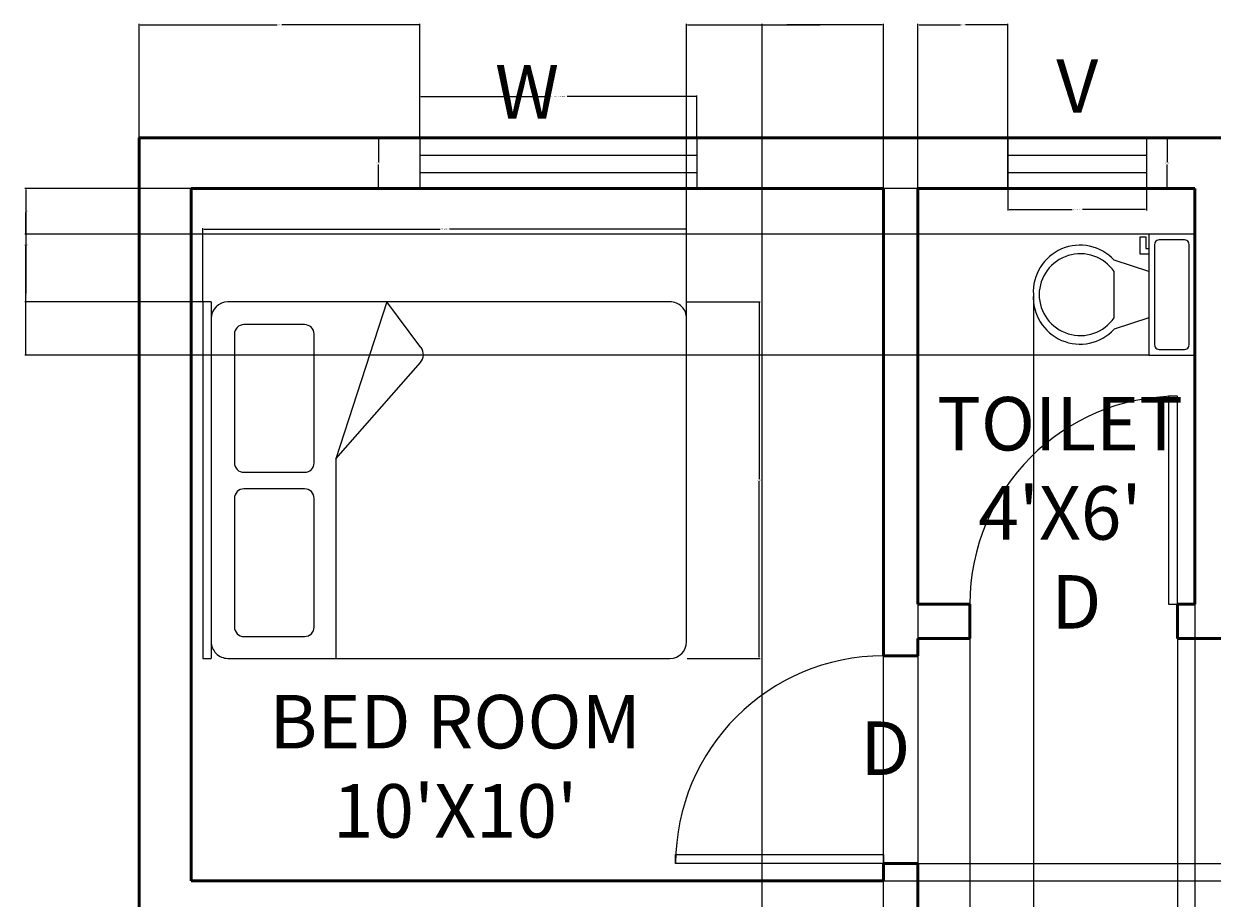
# Model space of a CAD drawing. Units: inches. Extents: x 1916 to 2328, y 785 to 1125.
# Tile 2 of 3: x 1916 to 2122, y 973 to 1125. Entities that reach past the tile are written whole.
import ezdxf

# ---------------------------------------------------------------- set-up
doc = ezdxf.new("R2010")
doc.units = ezdxf.units.IN
for name, color, linetype, lineweight in [('A-ANNO-DIMS', 2, 'Continuous', 18), ('A-ANNO-TEXT', 7, 'Continuous', 18), ('A-AREA-IDEN', 7, 'Continuous', 25), ('A-DOOR', 3, 'Continuous', 25), ('A-FLOR-FIXT', 9, 'Continuous', 18), ('A-FURN', 8, 'Continuous', 18), ('A-GLAZ', 4, 'Continuous', 18), ('A-WALL', 7, 'Continuous', 50)]:
    doc.layers.add(name, color=color, linetype=linetype, lineweight=lineweight)
doc.styles.get("Standard").update_dxf_attribs({"font": 'arial.ttf'})
doc.dimstyles.get("Standard").update_dxf_attribs({"dimtxt": 0.18, "dimasz": 0.18, "dimexe": 0.18, "dimexo": 0.0625, "dimgap": 0.09, "dimtad": 0, "dimtih": 1, "dimtoh": 1, "dimdec": 4, "dimzin": 0, "dimdsep": 46, "dimtxsty": 'Standard', "dimcen": 0.09, "dimadec": 0, "dimazin": 0, "dimtfac": 1, "dimtdec": 4, "dimtofl": 0, "dimtmove": 0, "dimatfit": 3, "dimfxl": 1, "dimtolj": 1, "dimtzin": 0, "dimarcsym": 0})

# ---------------------------------------------------------------- blocks, each defined once
blk = doc.blocks.new('*U2')
for p, q in [((0, 0), (0, -6)), ((40, 0), (40, -6))]:
    blk.add_line(p, q)
blk.add_lwpolyline([(0, 0), (0, 40), (1.75, 40), (1.75, 0)], close=True)
blk.add_arc((0, 0), 40, 0, 90)
blk = doc.blocks.new('*U8')
for p, q in [((0, 0), (0, -6)), ((-40, 0), (-40, -6))]:
    blk.add_line(p, q)
blk.add_lwpolyline([(0, 0), (0, 40), (-1.75, 40), (-1.75, 0)], close=True)
blk.add_arc((0, 0), 40, 90, 180)
blk = doc.blocks.new('A$C164346CA')
for p, q in [((0, 2.035), (0, 2)), ((1.5, 2.035), (0, 2.035)), ((1.5, 2), (0, 2)), ((1.5, 2), (1.5, 2.035)), ((0, 1.93), (0, 0.07)), ((0.6731, 1.9024), (0.1319, 1.9024)), ((1.364, 1.9024), (0.8228, 1.9024)), ((1.5, 0.07), (1.5, 1.93)), ((0.0919, 1.8624), (0.0919, 1.6069)), ((0.7131, 1.6069), (0.7131, 1.8624)), ((0.7828, 1.8624), (0.7828, 1.6069)), ((1.404, 1.6069), (1.404, 1.8624)), ((0.1319, 1.5669), (0.6731, 1.5669)), ((0.8228, 1.5669), (1.364, 1.5669)), ((0.8395, 1.4761), (0, 1.4761)), ((0.8395, 1.4761), (1.2448, 1.12)), ((1.5, 1.2611), (0.8395, 1.4761)), ((1.3077, 1.1175), (1.5, 1.2611)), ((0.07, 0), (1.43, 0))]:
    blk.add_line(p, q)
for centre, radius, start, end in [((0.07, 1.93), 0.07, 90, 180), ((1.43, 1.93), 0.07, 0, 90), ((0.1319, 1.8624), 0.04, 90, 180), ((0.6731, 1.8624), 0.04, 0, 90), ((0.8228, 1.8624), 0.04, 90, 180), ((1.364, 1.8624), 0.04, 0, 90), ((0.1319, 1.6069), 0.04, 180, 270), ((0.6731, 1.6069), 0.04, 270, 0), ((0.8228, 1.6069), 0.04, 180, 270), ((1.364, 1.6069), 0.04, 270, 0), ((1.2778, 1.1575), 0.05, 228.6958, 306.7579), ((0.07, 0.07), 0.07, 180, 270), ((1.43, 0.07), 0.07, 270, 0)]:
    blk.add_arc(centre, radius, start, end)
blk = doc.blocks.new('*U10')
for p, q in [((9.5, -6), (9.5, -2)), ((-8, -8.5), (-8, -8)), ((-7, -8), (-7, -9.5)), ((-4, -8), (-6, -14)), ((4, -8), (6, -14)), ((-10, -8.5), (-8, -8.5)), ((-10, -9.5), (-10, -8.5)), ((-7, -9.5), (-10, -9.5)), ((4, -14), (-4, -14))]:
    blk.add_line(p, q)
blk.add_lwpolyline([(10.5, -8), (10.5, 0), (-10.5, 0), (-10.5, -8)], close=True)
for points in [[(-9.5, -2), (-9.5, -6)], [(8.5, -1), (-8.5, -1)], [(-8.5, -7), (8.5, -7)]]:
    blk.add_lwpolyline(points)
for centre, radius, start, end in [((-8.625, -1.875), 0.8839, 81.8699, 188.1301), ((8.625, -1.875), 0.8839, 351.8699, 98.1301), ((-8.625, -6.125), 0.8839, 171.869898, 278.1301), ((8.625, -6.125), 0.8839, 261.8699, 8.1301), ((-0.4772, -19.9188), 8.0953, 133.01722, 273.38), ((0.0374, -19.8731), 7.127, 124.50543, 269.7), ((-0.0373, -19.8731), 7.127, 270.3, 55.4946), ((0.4773, -19.9188), 8.0953, 266.62, 46.9828)]:
    blk.add_arc(centre, radius, start, end)
blk = doc.blocks.new('WIN-48-JAMB-8_78')
for p, q in [((0, 8.78), (0, 0)), ((48, 8.78), (48, 0)), ((0, 5.78), (48, 5.78)), ((0, 2.78), (48, 2.78))]:
    blk.add_line(p, q)
blk = doc.blocks.new('VENT-24')
for p, q in [((0, 8.78), (0, 0)), ((24, 8.78), (24, 0)), ((0, 5.78), (24, 5.78)), ((0, 2.78), (24, 2.78))]:
    blk.add_line(p, q)
blk = doc.blocks.new('*D17')
at = {"layer": 'A-ANNO-DIMS', "color": 0, "lineweight": -2, "transparency": 16777216}
for p, q in [((1947.29, 1076.54), (1947.29, 1089.23)), ((1947.47, 1089.05), (1988.4, 1089.05)), ((2030.95, 1089.05), (1990.03, 1089.05)), ((2031.13, 1076.54), (2031.13, 1089.23))]:
    blk.add_line(p, q, dxfattribs=at)
at = {"layer": 'A-ANNO-DIMS', "color": 0, "transparency": 16777216}
for points in [[(1947.47, 1089.08), (1947.47, 1089.02), (1947.29, 1089.05)], [(2030.95, 1089.08), (2030.95, 1089.02), (2031.13, 1089.05)]]:
    blk.add_solid(points, dxfattribs=at)
at = {"layer": 'Defpoints', "color": 0, "transparency": 16777216}
for p in [(1947.29, 1089.05), (1947.29, 1076.48), (2031.13, 1076.48)]:
    blk.add_point(p, dxfattribs=at)
at = {"layer": 'A-ANNO-DIMS', "color": 0, "transparency": 16777216, "insert": (1989.21, 1089.05), "char_height": 0.18, "attachment_point": 5}
blk.add_mtext('\\A1;BED 84 TYP.', dxfattribs=at)
blk = doc.blocks.new('*D18')
at = {"layer": 'A-ANNO-DIMS', "color": 0, "lineweight": -2, "transparency": 16777216}
for p, q in [((2031.2, 1076.48), (2043.89, 1076.48)), ((2043.71, 1076.3), (2043.71, 1045.76)), ((2043.71, 1014.86), (2043.71, 1045.4)), ((2031.2, 1014.68), (2043.89, 1014.68))]:
    blk.add_line(p, q, dxfattribs=at)
at = {"layer": 'A-ANNO-DIMS', "color": 0, "transparency": 16777216}
for points in [[(2043.68, 1076.3), (2043.74, 1076.3), (2043.71, 1076.48)], [(2043.68, 1014.86), (2043.74, 1014.86), (2043.71, 1014.68)]]:
    blk.add_solid(points, dxfattribs=at)
at = {"layer": 'Defpoints', "color": 0, "transparency": 16777216}
for p in [(2031.13, 1076.48), (2043.71, 1076.48), (2031.13, 1014.68)]:
    blk.add_point(p, dxfattribs=at)
at = {"layer": 'A-ANNO-DIMS', "color": 0, "transparency": 16777216, "insert": (2043.71, 1045.58), "char_height": 0.18, "attachment_point": 5}
blk.add_mtext('\\A1;62 TYP.', dxfattribs=at)
blk = doc.blocks.new('*D19')
at = {"layer": 'A-ANNO-DIMS', "color": 0, "lineweight": -2, "transparency": 16777216}
for p, q in [((1984.91, 1104.94), (1984.91, 1112.26)), ((1985.09, 1112.08), (2007.42, 1112.08)), ((2032.73, 1112.08), (2010.4, 1112.08)), ((2032.91, 1104.94), (2032.91, 1112.26))]:
    blk.add_line(p, q, dxfattribs=at)
at = {"layer": 'A-ANNO-DIMS', "color": 0, "transparency": 16777216}
for points in [[(1985.09, 1112.11), (1985.09, 1112.05), (1984.91, 1112.08)], [(2032.73, 1112.11), (2032.73, 1112.05), (2032.91, 1112.08)]]:
    blk.add_solid(points, dxfattribs=at)
at = {"layer": 'Defpoints', "color": 0, "transparency": 16777216}
for p in [(2032.91, 1112.08), (1984.91, 1104.88), (2032.91, 1104.88)]:
    blk.add_point(p, dxfattribs=at)
at = {"layer": 'A-ANNO-DIMS', "color": 0, "transparency": 16777216, "insert": (2008.91, 1112.08), "char_height": 0.18, "attachment_point": 5}
blk.add_mtext('\\A1;WINDOW JAMB 48 TYP.', dxfattribs=at)
blk = doc.blocks.new('*D20')
at = {"layer": 'A-ANNO-DIMS', "color": 0, "lineweight": -2, "transparency": 16777216}
for p, q in [((1984.85, 1104.88), (1977.53, 1104.88)), ((1977.71, 1104.7), (1977.71, 1100.67)), ((1977.71, 1096.28), (1977.71, 1100.31)), ((1984.85, 1096.1), (1977.53, 1096.1))]:
    blk.add_line(p, q, dxfattribs=at)
at = {"layer": 'A-ANNO-DIMS', "color": 0, "transparency": 16777216}
for points in [[(1977.68, 1104.7), (1977.74, 1104.7), (1977.71, 1104.88)], [(1977.68, 1096.28), (1977.74, 1096.28), (1977.71, 1096.1)]]:
    blk.add_solid(points, dxfattribs=at)
at = {"layer": 'Defpoints', "color": 0, "transparency": 16777216}
for p in [(1977.71, 1104.88), (1984.91, 1104.88), (1984.91, 1096.1)]:
    blk.add_point(p, dxfattribs=at)
at = {"layer": 'A-ANNO-DIMS', "color": 0, "transparency": 16777216, "insert": (1977.71, 1100.49), "char_height": 0.18, "attachment_point": 5}
blk.add_mtext('\\A1;9 TYP.', dxfattribs=at)
blk = doc.blocks.new('*D21')
at = {"layer": 'A-ANNO-DIMS', "color": 0, "lineweight": -2, "transparency": 16777216}
for p, q in [((2086.83, 1096.04), (2086.83, 1092.32)), ((2110.83, 1096.04), (2110.83, 1092.32)), ((2087.01, 1092.5), (2097.93, 1092.5)), ((2110.65, 1092.5), (2099.73, 1092.5))]:
    blk.add_line(p, q, dxfattribs=at)
at = {"layer": 'A-ANNO-DIMS', "color": 0, "transparency": 16777216}
for points in [[(2087.01, 1092.53), (2087.01, 1092.47), (2086.83, 1092.5)], [(2110.65, 1092.53), (2110.65, 1092.47), (2110.83, 1092.5)]]:
    blk.add_solid(points, dxfattribs=at)
at = {"layer": 'Defpoints', "color": 0, "transparency": 16777216}
for p in [(2086.83, 1096.1), (2110.83, 1096.1), (2110.83, 1092.5)]:
    blk.add_point(p, dxfattribs=at)
at = {"layer": 'A-ANNO-DIMS', "color": 0, "transparency": 16777216, "insert": (2098.83, 1092.5), "char_height": 0.18, "attachment_point": 5}
blk.add_mtext('\\A1;VENT 24 TYP.', dxfattribs=at)
blk = doc.blocks.new('*D22')
at = {"layer": 'A-ANNO-DIMS', "color": 0, "lineweight": -2, "transparency": 16777216}
for p, q in [((2110.89, 1104.88), (2114.61, 1104.88)), ((2114.43, 1104.7), (2114.43, 1100.67)), ((2114.43, 1096.28), (2114.43, 1100.31)), ((2110.89, 1096.1), (2114.61, 1096.1))]:
    blk.add_line(p, q, dxfattribs=at)
at = {"layer": 'A-ANNO-DIMS', "color": 0, "transparency": 16777216}
for points in [[(2114.4, 1104.7), (2114.46, 1104.7), (2114.43, 1104.88)], [(2114.4, 1096.28), (2114.46, 1096.28), (2114.43, 1096.1)]]:
    blk.add_solid(points, dxfattribs=at)
at = {"layer": 'Defpoints', "color": 0, "transparency": 16777216}
for p in [(2110.83, 1104.88), (2114.43, 1104.88), (2110.83, 1096.1)]:
    blk.add_point(p, dxfattribs=at)
at = {"layer": 'A-ANNO-DIMS', "color": 0, "transparency": 16777216, "insert": (2114.43, 1100.49), "char_height": 0.18, "attachment_point": 5}
blk.add_mtext('\\A1;9 TYP.', dxfattribs=at)
blk = doc.blocks.new('*D31')
at = {"layer": 'A-ANNO-DIMS', "color": 0, "lineweight": -2, "transparency": 16777216}
for p, q in [((1936.23, 1104.94), (1936.23, 1124.67)), ((1936.41, 1124.49), (1960.17, 1124.49)), ((1984.73, 1124.49), (1960.97, 1124.49)), ((1984.91, 1104.94), (1984.91, 1124.67))]:
    blk.add_line(p, q, dxfattribs=at)
at = {"layer": 'A-ANNO-DIMS', "color": 0, "transparency": 16777216}
for points in [[(1936.41, 1124.52), (1936.41, 1124.46), (1936.23, 1124.49)], [(1984.73, 1124.52), (1984.73, 1124.46), (1984.91, 1124.49)]]:
    blk.add_solid(points, dxfattribs=at)
at = {"layer": 'Defpoints', "color": 0, "transparency": 16777216}
for p in [(1984.91, 1124.49), (1936.23, 1104.88), (1984.91, 1104.88)]:
    blk.add_point(p, dxfattribs=at)
at = {"layer": 'A-ANNO-DIMS', "color": 0, "transparency": 16777216, "insert": (1960.57, 1124.49), "char_height": 0.18, "attachment_point": 5}
blk.add_mtext('\\A1;48.68', dxfattribs=at)
blk = doc.blocks.new('*D32')
at = {"layer": 'A-ANNO-DIMS', "color": 0, "lineweight": -2, "transparency": 16777216}
for p, q in [((2071.23, 1096.16), (2071.23, 1124.67)), ((2071.41, 1124.49), (2078.58, 1124.49)), ((2086.65, 1124.49), (2079.49, 1124.49)), ((2086.83, 1096.16), (2086.83, 1124.67))]:
    blk.add_line(p, q, dxfattribs=at)
at = {"layer": 'A-ANNO-DIMS', "color": 0, "transparency": 16777216}
for points in [[(2071.41, 1124.52), (2071.41, 1124.46), (2071.23, 1124.49)], [(2086.65, 1124.52), (2086.65, 1124.46), (2086.83, 1124.49)]]:
    blk.add_solid(points, dxfattribs=at)
at = {"layer": 'Defpoints', "color": 0, "transparency": 16777216}
for p in [(2086.83, 1124.49), (2071.23, 1096.1), (2086.83, 1096.1)]:
    blk.add_point(p, dxfattribs=at)
at = {"layer": 'A-ANNO-DIMS', "color": 0, "transparency": 16777216, "insert": (2079.03, 1124.49), "char_height": 0.18, "attachment_point": 5}
blk.add_mtext('\\A1;15.597', dxfattribs=at)
blk = doc.blocks.new('*D43')
at = {"layer": 'A-ANNO-DIMS', "color": 0, "lineweight": -2, "transparency": 16777216}
for p, q in [((2044.24, 834.38), (2044.24, 1124.67)), ((2044.42, 1124.49), (2054.27, 1124.49)), ((2065.05, 1124.49), (2055.2, 1124.49)), ((2065.23, 837.94), (2065.23, 1124.67))]:
    blk.add_line(p, q, dxfattribs=at)
at = {"layer": 'A-ANNO-DIMS', "color": 0, "transparency": 16777216}
for points in [[(2044.42, 1124.52), (2044.42, 1124.46), (2044.24, 1124.49)], [(2065.05, 1124.52), (2065.05, 1124.46), (2065.23, 1124.49)]]:
    blk.add_solid(points, dxfattribs=at)
at = {"layer": 'Defpoints', "color": 0, "transparency": 16777216}
for p in [(2065.23, 1124.49), (2065.23, 837.88), (2044.24, 834.32)]:
    blk.add_point(p, dxfattribs=at)
at = {"layer": 'A-ANNO-DIMS', "color": 0, "transparency": 16777216, "insert": (2054.74, 1124.49), "char_height": 0.18, "attachment_point": 5}
blk.add_mtext('\\A1;20.992', dxfattribs=at)
blk = doc.blocks.new('*D46')
at = {"layer": 'A-ANNO-DIMS', "color": 0, "lineweight": -2, "transparency": 16777216}
for p, q in [((2111.17, 1088.22), (1916.44, 1088.22)), ((1916.62, 1088.04), (1916.62, 1077.9)), ((1916.62, 1067.4), (1916.62, 1077.54)), ((2111.17, 1067.22), (1916.44, 1067.22))]:
    blk.add_line(p, q, dxfattribs=at)
at = {"layer": 'A-ANNO-DIMS', "color": 0, "transparency": 16777216}
for points in [[(1916.59, 1088.04), (1916.65, 1088.04), (1916.62, 1088.22)], [(1916.59, 1067.4), (1916.65, 1067.4), (1916.62, 1067.22)]]:
    blk.add_solid(points, dxfattribs=at)
at = {"layer": 'Defpoints', "color": 0, "transparency": 16777216}
for p in [(1916.62, 1088.22), (2111.23, 1088.22), (2111.23, 1067.22)]:
    blk.add_point(p, dxfattribs=at)
at = {"layer": 'A-ANNO-DIMS', "color": 0, "transparency": 16777216, "insert": (1916.62, 1077.72), "char_height": 0.18, "attachment_point": 5}
blk.add_mtext('\\A1;21', dxfattribs=at)
blk = doc.blocks.new('*D47')
at = {"layer": 'A-ANNO-DIMS', "color": 0, "lineweight": -2, "transparency": 16777216}
for p, q in [((2091.23, 1077.66), (2091.23, 785.08)), ((2119.23, 1067.16), (2119.23, 785.08)), ((2091.41, 785.26), (2105.01, 785.26)), ((2119.05, 785.26), (2105.45, 785.26))]:
    blk.add_line(p, q, dxfattribs=at)
at = {"layer": 'A-ANNO-DIMS', "color": 0, "transparency": 16777216}
for points in [[(2091.41, 785.29), (2091.41, 785.23), (2091.23, 785.26)], [(2119.05, 785.29), (2119.05, 785.23), (2119.23, 785.26)]]:
    blk.add_solid(points, dxfattribs=at)
at = {"layer": 'Defpoints', "color": 0, "transparency": 16777216}
for p in [(2091.23, 1077.72), (2119.23, 1067.22), (2119.23, 785.26)]:
    blk.add_point(p, dxfattribs=at)
at = {"layer": 'A-ANNO-DIMS', "color": 0, "transparency": 16777216, "insert": (2105.23, 785.26), "char_height": 0.18, "attachment_point": 5}
blk.add_mtext('\\A1;28', dxfattribs=at)
blk = doc.blocks.new('*D48')
at = {"layer": 'A-ANNO-DIMS', "color": 0, "lineweight": -2, "transparency": 16777216}
for p, q in [((2119.17, 1096.1), (1916.44, 1096.1)), ((1916.62, 1095.92), (1916.62, 1092.34)), ((1916.62, 1088.4), (1916.62, 1091.98)), ((2119.17, 1088.22), (1916.44, 1088.22))]:
    blk.add_line(p, q, dxfattribs=at)
at = {"layer": 'A-ANNO-DIMS', "color": 0, "transparency": 16777216}
for points in [[(1916.59, 1095.92), (1916.65, 1095.92), (1916.62, 1096.1)], [(1916.59, 1088.4), (1916.65, 1088.4), (1916.62, 1088.22)]]:
    blk.add_solid(points, dxfattribs=at)
at = {"layer": 'Defpoints', "color": 0, "transparency": 16777216}
for p in [(1916.62, 1096.1), (2119.23, 1096.1), (2119.23, 1088.22)]:
    blk.add_point(p, dxfattribs=at)
at = {"layer": 'A-ANNO-DIMS', "color": 0, "transparency": 16777216, "insert": (1916.62, 1092.16), "char_height": 0.18, "attachment_point": 5}
blk.add_mtext('\\A1;7.88', dxfattribs=at)
blk = doc.blocks.new('*D50')
at = {"layer": 'A-ANNO-DIMS', "color": 0, "lineweight": -2, "transparency": 16777216}
for p, q in [((2071.23, 1024.04), (2071.23, 785.08)), ((2080.23, 1024.04), (2080.23, 785.08)), ((2071.41, 785.26), (2075.58, 785.26)), ((2080.05, 785.26), (2075.88, 785.26))]:
    blk.add_line(p, q, dxfattribs=at)
at = {"layer": 'A-ANNO-DIMS', "color": 0, "transparency": 16777216}
for points in [[(2071.41, 785.29), (2071.41, 785.23), (2071.23, 785.26)], [(2080.05, 785.29), (2080.05, 785.23), (2080.23, 785.26)]]:
    blk.add_solid(points, dxfattribs=at)
at = {"layer": 'Defpoints', "color": 0, "transparency": 16777216}
for p in [(2071.23, 1024.1), (2080.23, 1024.1), (2080.23, 785.26)]:
    blk.add_point(p, dxfattribs=at)
at = {"layer": 'A-ANNO-DIMS', "color": 0, "transparency": 16777216, "insert": (2075.73, 785.26), "char_height": 0.18, "attachment_point": 5}
blk.add_mtext('\\A1;9', dxfattribs=at)
blk = doc.blocks.new('*D51')
at = {"layer": 'A-ANNO-DIMS', "color": 0, "lineweight": -2, "transparency": 16777216}
for p, q in [((2080.23, 1024.04), (2080.23, 785.08)), ((2116.23, 1024.04), (2116.23, 785.08)), ((2080.41, 785.26), (2098.01, 785.26)), ((2116.05, 785.26), (2098.45, 785.26))]:
    blk.add_line(p, q, dxfattribs=at)
at = {"layer": 'A-ANNO-DIMS', "color": 0, "transparency": 16777216}
for points in [[(2080.41, 785.29), (2080.41, 785.23), (2080.23, 785.26)], [(2116.05, 785.29), (2116.05, 785.23), (2116.23, 785.26)]]:
    blk.add_solid(points, dxfattribs=at)
at = {"layer": 'Defpoints', "color": 0, "transparency": 16777216}
for p in [(2080.23, 1024.1), (2116.23, 1024.1), (2116.23, 785.26)]:
    blk.add_point(p, dxfattribs=at)
at = {"layer": 'A-ANNO-DIMS', "color": 0, "transparency": 16777216, "insert": (2098.23, 785.26), "char_height": 0.18, "attachment_point": 5}
blk.add_mtext('\\A1;36', dxfattribs=at)
blk = doc.blocks.new('*D54')
at = {"layer": 'A-ANNO-DIMS', "color": 0, "lineweight": -2, "transparency": 16777216}
for p, q in [((2065.3, 979.1), (2328.03, 979.1)), ((2327.85, 978.92), (2327.85, 977.78)), ((2327.85, 976.28), (2327.85, 977.42)), ((2065.3, 976.1), (2328.03, 976.1))]:
    blk.add_line(p, q, dxfattribs=at)
at = {"layer": 'A-ANNO-DIMS', "color": 0, "transparency": 16777216}
for points in [[(2327.82, 978.92), (2327.88, 978.92), (2327.85, 979.1)], [(2327.82, 976.28), (2327.88, 976.28), (2327.85, 976.1)]]:
    blk.add_solid(points, dxfattribs=at)
at = {"layer": 'Defpoints', "color": 0, "transparency": 16777216}
for p in [(2065.23, 979.1), (2327.85, 979.1), (2065.23, 976.1)]:
    blk.add_point(p, dxfattribs=at)
at = {"layer": 'A-ANNO-DIMS', "color": 0, "transparency": 16777216, "insert": (2327.85, 977.6), "char_height": 0.18, "attachment_point": 5}
blk.add_mtext('\\A1;3', dxfattribs=at)
blk = doc.blocks.new('*D55')
at = {"layer": 'A-ANNO-DIMS', "color": 0, "lineweight": -2, "transparency": 16777216}
for p, q in [((2031.13, 1073.66), (2031.13, 1124.67)), ((2031.31, 1124.49), (2047.88, 1124.49)), ((2065.05, 1124.49), (2048.49, 1124.49)), ((2065.23, 1096.16), (2065.23, 1124.67))]:
    blk.add_line(p, q, dxfattribs=at)
at = {"layer": 'A-ANNO-DIMS', "color": 0, "transparency": 16777216}
for points in [[(2031.31, 1124.52), (2031.31, 1124.46), (2031.13, 1124.49)], [(2065.05, 1124.52), (2065.05, 1124.46), (2065.23, 1124.49)]]:
    blk.add_solid(points, dxfattribs=at)
at = {"layer": 'Defpoints', "color": 0, "transparency": 16777216}
for p in [(2065.23, 1124.49), (2065.23, 1096.1), (2031.13, 1073.59)]:
    blk.add_point(p, dxfattribs=at)
at = {"layer": 'A-ANNO-DIMS', "color": 0, "transparency": 16777216, "insert": (2048.18, 1124.49), "char_height": 0.18, "attachment_point": 5}
blk.add_mtext('\\A1;34.1', dxfattribs=at)
blk = doc.blocks.new('*D56')
at = {"layer": 'A-ANNO-DIMS', "color": 0, "lineweight": -2, "transparency": 16777216}
for p, q in [((1945.17, 1096.1), (1916.44, 1096.1)), ((1916.62, 1095.92), (1916.62, 1086.47)), ((1916.62, 1076.66), (1916.62, 1086.11)), ((1947.23, 1076.48), (1916.44, 1076.48))]:
    blk.add_line(p, q, dxfattribs=at)
at = {"layer": 'A-ANNO-DIMS', "color": 0, "transparency": 16777216}
for points in [[(1916.59, 1095.92), (1916.65, 1095.92), (1916.62, 1096.1)], [(1916.59, 1076.66), (1916.65, 1076.66), (1916.62, 1076.48)]]:
    blk.add_solid(points, dxfattribs=at)
at = {"layer": 'Defpoints', "color": 0, "transparency": 16777216}
for p in [(1916.62, 1096.1), (1945.23, 1096.1), (1947.29, 1076.48)]:
    blk.add_point(p, dxfattribs=at)
at = {"layer": 'A-ANNO-DIMS', "color": 0, "transparency": 16777216, "insert": (1916.62, 1086.29), "char_height": 0.18, "attachment_point": 5}
blk.add_mtext('\\A1;19.623', dxfattribs=at)

msp = doc.modelspace()

# ---------------------------------------------------------------- linework, layer by layer
at = {"layer": 'A-WALL'}
for p, q in [((1936.2334, 1104.8797), (2308.2334, 1104.8797)), ((1936.2334, 804.8797), (1936.2334, 1104.8797)), ((1945.2334, 1096.1011), (2065.2334, 1096.1011)), ((1945.2334, 976.1011), (1945.2334, 1096.1011)), ((2065.2334, 1015.1011), (2065.2334, 1096.1011)), ((2071.2334, 1096.1011), (2119.2334, 1096.1011)), ((2071.2334, 1024.1011), (2071.2334, 1096.1011)), ((2119.2334, 1024.1011), (2119.2334, 1096.1011)), ((2071.2334, 1024.1011), (2080.2334, 1024.1011)), ((2080.2334, 1024.1011), (2080.2334, 1018.1011)), ((2116.2334, 1024.1011), (2116.2334, 1018.1011)), ((2116.2334, 1024.1011), (2119.2334, 1024.1011)), ((2071.2334, 1018.1011), (2080.2334, 1018.1011)), ((2071.2334, 1015.1011), (2071.2334, 1018.1011)), ((2116.2334, 1018.1011), (2173.2334, 1018.1011)), ((2071.2334, 1015.1011), (2065.2334, 1015.1011)), ((2065.2334, 976.1011), (2065.2334, 979.1011)), ((2071.2334, 979.1011), (2065.2334, 979.1011)), ((2071.2334, 979.1011), (2065.2334, 979.1011)), ((2071.2334, 970.1011), (2071.2334, 979.1011)), ((1945.2334, 976.1011), (2065.2334, 976.1011))]:
    msp.add_line(p, q, dxfattribs=at)

# ---------------------------------------------------------------- block references
at = {"layer": 'A-DOOR', "xscale": 0.9, "yscale": 0.9, "zscale": 0.9}
msp.add_blockref('*U8', (2116.2334, 1024.1011), dxfattribs=at)
at = {"layer": 'A-DOOR', "xscale": 0.900000000000009, "yscale": 0.900000000000009, "zscale": 0.900000000000009, "rotation": 90}
msp.add_blockref('*U2', (2065.2334, 979.1011), dxfattribs=at)
at = {"layer": 'A-FLOR-FIXT', "rotation": 270}
msp.add_blockref('*U10', (2119.2334, 1077.7207), dxfattribs=at)
at = {"layer": 'A-FURN', "xscale": 41.2001878286395, "yscale": 41.2001878286395, "zscale": 41.2001878286395, "rotation": 89.99999999999999}
msp.add_blockref('A$C164346CA', (2031.1339, 1014.6778), dxfattribs=at)
at = {"layer": 'A-GLAZ'}
for name, p in [('WIN-48-JAMB-8_78', (1984.9113, 1096.1011)), ('VENT-24', (2086.8308, 1096.1011))]:
    msp.add_blockref(name, p, dxfattribs=at)

# ---------------------------------------------------------------- texts
at = {"layer": 'A-ANNO-TEXT', "char_height": 9.27346, "attachment_point": 1}
for s, insert in [('\\pxqc;V', (2093.4424, 1118.5258)), ('\\pxqc;W', (1998.0842, 1117.5066)), ('\\pxqc;D', (2093.2815, 1029.1035)), ('\\pxqc;D', (2060.1656, 1003.7355))]:
    msp.add_mtext_dynamic_manual_height_columns(s, width=10.785675, gutter_width=46.3673, heights=[0], dxfattribs=dict(at, insert=insert))
at = {"layer": 'A-AREA-IDEN', "char_height": 9.273456, "attachment_point": 1}
for s, width, insert in [("\\pxqc;TOILET\\P4'X6'", 10.785675, (2090.4525, 1059.9863)), ("\\pxqc;BED ROOM\\P10'X10'", 69.285743, (1956.3687, 1008.3378))]:
    msp.add_mtext_dynamic_manual_height_columns(s, width=width, gutter_width=46.3673, heights=[0], dxfattribs=dict(at, insert=insert))

# ---------------------------------------------------------------- dimensions: what is measured, and where the dimension line sits
at = {"layer": 'A-ANNO-DIMS'}
for base, p1, p2, override, picture, middle in [((1984.9113, 1124.4947), (1936.2334, 1104.8797), (1984.9113, 1104.8797), {"dimdec": 2, "dimlfac": 1, "dimrnd": 0, "dimzin": 0, "dimdsep": 46, "dimlunit": 2}, '*D31', (1960.5723, 1124.4947)), ((2065.2334, 1124.4947), (2031.1339, 1073.5941), (2065.2334, 1096.1011), {"dimdec": 1, "dimlfac": 1, "dimrnd": 0, "dimzin": 0, "dimdsep": 46, "dimlunit": 2}, '*D55', (2048.1836, 1124.4947)), ((2065.2334, 1124.4947), (2044.241, 834.3209), (2065.2334, 837.8797), {"dimdec": 3, "dimlfac": 1, "dimrnd": 0, "dimzin": 0, "dimdsep": 46, "dimlunit": 2}, '*D43', (2054.7372, 1124.4947)), ((2086.8308, 1124.4947), (2071.2334, 1096.1011), (2086.8308, 1096.1011), {"dimdec": 3, "dimlfac": 1, "dimrnd": 0, "dimzin": 0, "dimdsep": 46, "dimlunit": 2}, '*D32', (2079.0321, 1124.4947)), ((2119.2334, 785.2647), (2091.2334, 1077.7207), (2119.2334, 1067.2207), {"dimdec": 0, "dimlfac": 1, "dimrnd": 0, "dimzin": 0, "dimdsep": 46, "dimlunit": 2}, '*D47', (2105.2334, 785.2647)), ((2080.2334, 785.2647), (2071.2334, 1024.1011), (2080.2334, 1024.1011), {"dimdec": 0, "dimlfac": 1, "dimrnd": 0, "dimzin": 0, "dimdsep": 46, "dimlunit": 2}, '*D50', (2075.7334, 785.2647)), ((2116.2334, 785.2647), (2080.2334, 1024.1011), (2116.2334, 1024.1011), {"dimdec": 0, "dimlfac": 1, "dimrnd": 0, "dimzin": 0, "dimdsep": 46, "dimlunit": 2}, '*D51', (2098.2334, 785.2647))]:
    dim = msp.add_linear_dim(base=base, p1=p1, p2=p2, dimstyle='Standard', override=override, dxfattribs=at)
    dim.commit()
    dim.dimension.update_dxf_attribs({"geometry": picture, "text_midpoint": middle})
for base, p1, p2, text, picture, middle in [((2032.9113, 1112.0797), (1984.9113, 1104.8797), (2032.9113, 1104.8797), 'WINDOW JAMB <> TYP.', '*D19', (2008.9113, 1112.0797)), ((2110.8308, 1092.5011), (2086.8308, 1096.1011), (2110.8308, 1096.1011), 'VENT <> TYP.', '*D21', (2098.8308, 1092.5011))]:
    dim = msp.add_linear_dim(base=base, p1=p1, p2=p2, text=text, dimstyle='Standard', override={"dimdec": 0, "dimlfac": 1, "dimrnd": 0, "dimzin": 0, "dimdsep": 46, "dimlunit": 2}, dxfattribs=at)
    dim.commit()
    dim.dimension.update_dxf_attribs({"geometry": picture, "text_midpoint": middle})
for base, p1, p2, angle, text, picture, middle in [((1977.7113, 1104.8797), (1984.9113, 1096.1011), (1984.9113, 1104.8797), 90, '<> TYP.', '*D20', (1977.7113, 1100.4904)), ((2114.4308, 1104.8797), (2110.8308, 1096.1011), (2110.8308, 1104.8797), 90, '<> TYP.', '*D22', (2114.4308, 1100.4904)), ((1947.2915, 1089.0544), (2031.1339, 1076.4781), (1947.2915, 1076.4781), 180, 'BED <> TYP.', '*D17', (1989.2127, 1089.0544)), ((2043.7102, 1076.4781), (2031.1339, 1014.6778), (2031.1339, 1076.4781), 90, '<> TYP.', '*D18', (2043.7102, 1045.5779))]:
    dim = msp.add_linear_dim(base=base, p1=p1, p2=p2, angle=angle, text=text, dimstyle='Standard', override={"dimdec": 0, "dimlfac": 1, "dimrnd": 0, "dimzin": 0, "dimdsep": 46, "dimlunit": 2}, dxfattribs=at)
    dim.commit()
    dim.dimension.update_dxf_attribs({"geometry": picture, "text_midpoint": middle})
for base, p1, p2, override, picture, middle in [((1916.6184, 1096.1011), (1947.2915, 1076.4781), (1945.2334, 1096.1011), {"dimdec": 3, "dimlfac": 1, "dimrnd": 0, "dimzin": 0, "dimdsep": 46, "dimlunit": 2}, '*D56', (1916.6184, 1086.2896)), ((1916.6184, 1096.1011), (2119.2334, 1088.2207), (2119.2334, 1096.1011), {"dimdec": 2, "dimlfac": 1, "dimrnd": 0, "dimzin": 0, "dimdsep": 46, "dimlunit": 2}, '*D48', (1916.6184, 1092.1609)), ((1916.6184, 1088.2207), (2111.2334, 1067.2207), (2111.2334, 1088.2207), {"dimdec": 0, "dimlfac": 1, "dimrnd": 0, "dimzin": 0, "dimdsep": 46, "dimlunit": 2}, '*D46', (1916.6184, 1077.7207)), ((2327.8484, 979.1011), (2065.2334, 976.1011), (2065.2334, 979.1011), {"dimdec": 0, "dimlfac": 1, "dimrnd": 0, "dimzin": 0, "dimdsep": 46, "dimlunit": 2}, '*D54', (2327.8484, 977.6011))]:
    dim = msp.add_linear_dim(base=base, p1=p1, p2=p2, angle=90, dimstyle='Standard', override=override, dxfattribs=at)
    dim.commit()
    dim.dimension.update_dxf_attribs({"geometry": picture, "text_midpoint": middle})

doc.saveas('drawing.dxf')
